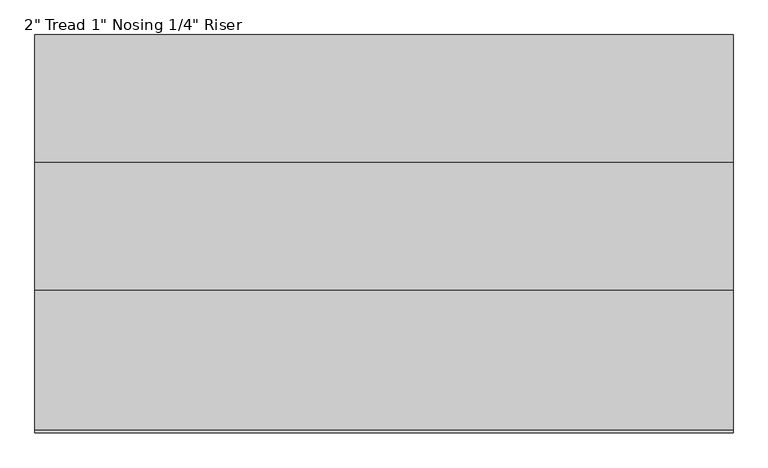
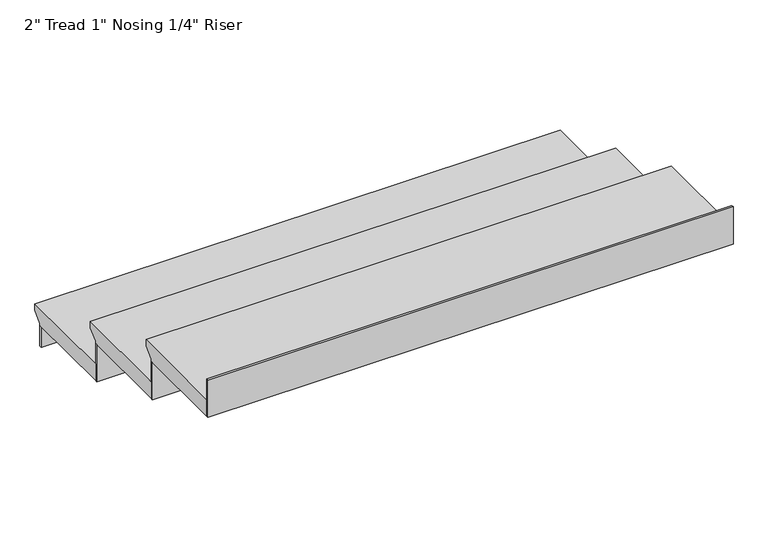
"""IFC4 building model written with IfcOpenShell, lengths in millimetres: stair flight geometry."""

from ifc_helpers import new_model, si_unit, frame, origin, place, context, project, spatial, polyline, outline, extrude, source, transform, mapped, element, save


def stair_flight_d6b1375f(model_context):
    return source(origin(), model_context, "Body", "SweptSolid", [
        extrude(outline(polyline([(-11606.7027976, 571.5), (-11301.9027976, 571.5), (-11301.9027976, 552.45), (-11327.3027976, 527.05), (-11327.3027976, 520.7), (-11606.7027976, 520.7), (-11606.7027976, 571.5)])), frame((-17069.368705, 0.0, 0.0), z_axis=(1.0, 0.0, 0.0), x_axis=(0.0, 1.0, 0.0)), (0.0, 0.0, 1.0), 1524.0),
        extrude(outline(polyline([(-17069.368705, -11333.6527976), (-17069.368705, -11327.3027976), (-15545.368705, -11327.3027976), (-15545.368705, -11333.6527976), (-17069.368705, -11333.6527976)])), frame((0.0, 0.0, 457.2), z_axis=(0.0, 0.0, 1.0), x_axis=(1.0, 0.0, 0.0)), (0.0, 0.0, 1.0), 63.5),
        extrude(outline(polyline([(-17069.368705, -11613.0527976), (-17069.368705, -11606.7027976), (-15545.368705, -11606.7027976), (-15545.368705, -11613.0527976), (-17069.368705, -11613.0527976)])), frame((0.0, 0.0, 520.7), z_axis=(0.0, 0.0, 1.0), x_axis=(1.0, 0.0, 0.0)), (0.0, 0.0, 1.0), 114.3),
        extrude(outline(polyline([(-11886.1027976, 685.8), (-11581.3027976, 685.8), (-11581.3027976, 666.75), (-11606.7027976, 641.35), (-11606.7027976, 635.0), (-11886.1027976, 635.0), (-11886.1027976, 685.8)])), frame((-17069.368705, 0.0, 0.0), z_axis=(1.0, 0.0, 0.0), x_axis=(0.0, 1.0, 0.0)), (0.0, 0.0, 1.0), 1524.0),
        extrude(outline(polyline([(-17069.368705, -11892.4527976), (-17069.368705, -11886.1027976), (-15545.368705, -11886.1027976), (-15545.368705, -11892.4527976), (-17069.368705, -11892.4527976)])), frame((0.0, 0.0, 635.0), z_axis=(0.0, 0.0, 1.0), x_axis=(1.0, 0.0, 0.0)), (0.0, 0.0, 1.0), 114.3),
        extrude(outline(polyline([(-17069.368705, -12171.8527976), (-17069.368705, -12165.5027976), (-15545.368705, -12165.5027976), (-15545.368705, -12171.8527976), (-17069.368705, -12171.8527976)])), frame((0.0, 0.0, 749.3), z_axis=(0.0, 0.0, 1.0), x_axis=(1.0, 0.0, 0.0)), (0.0, 0.0, 1.0), 114.3),
        extrude(outline(polyline([(-12165.5027976, 800.1), (-11860.7027976, 800.1), (-11860.7027976, 781.05), (-11886.1027976, 755.65), (-11886.1027976, 749.3), (-12165.5027976, 749.3), (-12165.5027976, 800.1)])), frame((-17069.368705, 0.0, 0.0), z_axis=(1.0, 0.0, 0.0), x_axis=(0.0, 1.0, 0.0)), (0.0, 0.0, 1.0), 1524.0),
    ])


if __name__ == "__main__":
    model = new_model("IFC4")
    model_context = context("Model", 3, world=origin())
    ifc_project = project(units=[si_unit("LENGTHUNIT", "METRE", prefix="MILLI")], contexts=[model_context])
    site = spatial("IfcSite", under=ifc_project)
    building = spatial("IfcBuilding", under=site)
    placement = place(None, origin())
    stair_flight_shape = stair_flight_d6b1375f(model_context)
    element("IfcStairFlight", 1, ObjectType="2\" Tread 1\" Nosing 1/4\" Riser", at=placement, inside=building, context=model_context, shape_type="MappedRepresentation", body=[
        mapped(stair_flight_shape, transform((0.0, 0.0, 0.0), x_axis=(1.0, 0.0, 0.0), y_axis=(0.0, 1.0, 0.0), z_axis=(0.0, 0.0, 1.0))),
    ])
    save(model, "model.ifc")
